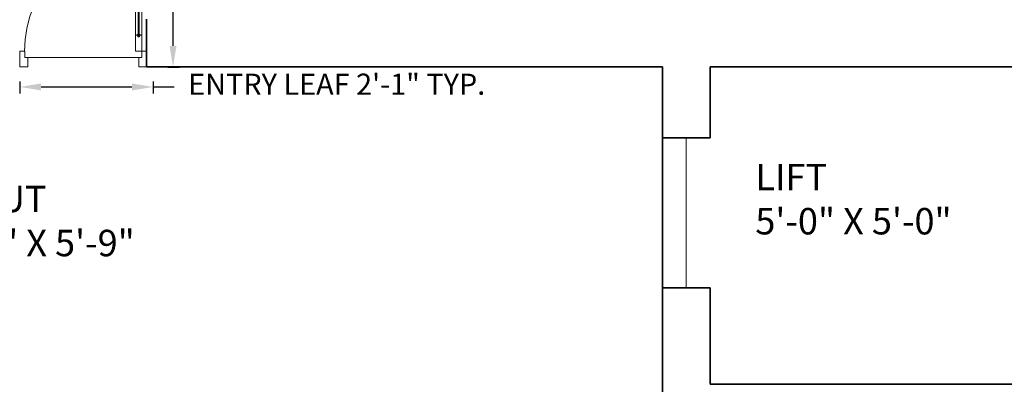
# Model space of a CAD drawing. Units: inches. Extents: x -638 to 186, y -762 to 59.
# Tile 3 of 31: x -287 to -100, y -608 to -539. Entities that reach past the tile are written whole.
import ezdxf

# ---------------------------------------------------------------- set-up
doc = ezdxf.new("R2010")
doc.units = ezdxf.units.IN
for name, color, linetype, lineweight in [('A-ANNO-DIMS', 2, 'Continuous', 18), ('A-AREA-IDEN', 1, 'Continuous', 18), ('A-DOOR', 3, 'Continuous', 18), ('wall', 7, 'Continuous', 35)]:
    doc.layers.add(name, color=color, linetype=linetype, lineweight=lineweight)
doc.styles.get("Standard").update_dxf_attribs({"font": 'arial.ttf'})
doc.dimstyles.new('ISO-25', dxfattribs={"dimtxt": 4, "dimasz": 4, "dimexe": 1.25, "dimexo": 0.625, "dimtad": 0, "dimlunit": 4, "dimtxsty": 'Standard', "dimcen": 2.5, "dimclrt": 256, "dimadec": 0, "dimazin": 0, "dimtfac": 1, "dimtmove": 0, "dimatfit": 3, "dimfxl": 1, "dimfxlon": 1, "dimarcsym": 0})

# ---------------------------------------------------------------- blocks, each defined once
blk = doc.blocks.new('DOOR-ENTRY-24IN-LEAF')
for p, q in [((22.38, 22.44), (22.37, 5.69)), ((22.45, 22.44), (22.45, 5.69)), ((22.53, 22.44), (22.52, 5.69)), ((21.85, 22.14), (21.85, 5.99)), ((23.05, 22.14), (23.04, 5.99)), ((1.5, 1.8), (22.44, 1.8))]:
    blk.add_line(p, q)
for points in [[(21.11, 23.03), (19.91, 22.91, -0.443716), (19.75, 23.06), (19.75, 24.22, -0.443716), (19.91, 24.37), (21.11, 24.25, -0.385314), (21.24, 24.1), (21.24, 23.18, -0.385314)], [(23.79, 23.03), (24.99, 22.91, 0.443716), (25.15, 23.06), (25.16, 24.22, 0.443716), (24.99, 24.37), (23.79, 24.25, 0.385314), (23.66, 24.1), (23.66, 23.18, 0.385314)]]:
    blk.add_lwpolyline(points, format="xyb", close=True)
for points in [[(22.3, 22.14), (21.85, 22.14), (21.85, 25.14), (23.05, 25.14), (23.05, 22.14), (22.6, 22.14), (22.6, 22.44), (22.3, 22.44), (22.3, 22.14)], [(22.3, 5.99), (21.85, 5.99), (21.85, 2.99), (23.04, 2.99), (23.04, 5.99), (22.59, 5.99), (22.59, 5.69), (22.3, 5.69), (22.3, 5.99)], [(0.9, 3), (0.9, 1.8), (1.5, 1.8), (1.5, 0.01), (0, 0.01), (0, 3), (0.9, 3)], [(23.04, 2.99), (23.04, 1.8), (22.44, 1.8), (22.44, 0), (23.94, 0), (23.94, 2.99), (23.04, 2.99)]]:
    blk.add_lwpolyline(points)
for points in [[(21.85, 23.49), (21.24, 23.49), (21.24, 23.79), (21.85, 23.79)], [(23.05, 23.49), (23.66, 23.49), (23.66, 23.79), (23.05, 23.79)]]:
    blk.add_lwpolyline(points, close=True)
for centre, radius, start, end in [((23.1, 2.97), 22.21, 93.2293, 179.917), ((22.36, 22.17), 0.247, 186.4162, 273.2718), ((22.54, 22.17), 0.247, 266.6922, 353.5478), ((22.36, 5.96), 0.247, 86.6922, 173.5478), ((22.53, 5.96), 0.247, 6.4162, 93.2718)]:
    blk.add_arc(centre, radius, start, end)
blk = doc.blocks.new('*D29')
at = {"layer": 'A-ANNO-DIMS', "color": 0, "lineweight": -2, "transparency": 16777216}
for p, q in [((-286.47, -550.82), (-286.47, -553.07)), ((-261.32, -550.82), (-261.32, -553.07)), ((-282.47, -551.82), (-265.32, -551.82)), ((-261.32, -551.82), (-257.32, -551.82))]:
    blk.add_line(p, q, dxfattribs=at)
at = {"layer": 'A-ANNO-DIMS', "color": 0, "lineweight": 30, "transparency": 16777216}
for points in [[(-282.47, -551.15), (-282.47, -552.49), (-286.47, -551.82)], [(-265.32, -551.15), (-265.32, -552.49), (-261.32, -551.82)]]:
    blk.add_solid(points, dxfattribs=at)
at = {"layer": 'Defpoints', "color": 0, "lineweight": 30, "transparency": 16777216}
for p in [(-286.47, -548.05), (-261.32, -548.05), (-261.32, -551.82)]:
    blk.add_point(p, dxfattribs=at)
at = {"layer": 'A-ANNO-DIMS', "transparency": 16777216, "insert": (-226.6, -551.82), "char_height": 4, "attachment_point": 5}
blk.add_mtext('ENTRY LEAF 2\'-1" TYP.', dxfattribs=at)
blk = doc.blocks.new('*D30')
at = {"layer": 'A-ANNO-DIMS', "color": 0, "lineweight": -2, "transparency": 16777216}
for p, q in [((-257.54, -522.91), (-257.54, -518.91)), ((-258.54, -522.91), (-256.29, -522.91)), ((-257.54, -544.05), (-257.54, -526.91)), ((-258.54, -548.05), (-256.29, -548.05))]:
    blk.add_line(p, q, dxfattribs=at)
at = {"layer": 'A-ANNO-DIMS', "color": 0, "lineweight": 30, "transparency": 16777216}
for points in [[(-258.21, -526.91), (-256.88, -526.91), (-257.54, -522.91)], [(-258.21, -544.05), (-256.88, -544.05), (-257.54, -548.05)]]:
    blk.add_solid(points, dxfattribs=at)
at = {"layer": 'Defpoints', "color": 0, "lineweight": 30, "transparency": 16777216}
for p in [(-261.32, -522.91), (-257.54, -522.91), (-261.32, -548.05)]:
    blk.add_point(p, dxfattribs=at)
at = {"layer": 'A-ANNO-DIMS', "transparency": 16777216, "insert": (-257.54, -506.06), "char_height": 4, "attachment_point": 5, "rotation": 90}
blk.add_mtext('2\'-1" TYP.', dxfattribs=at)
blk = doc.blocks.new('*D39')
at = {"layer": 'A-ANNO-DIMS', "color": 0, "lineweight": -2, "transparency": 16777216}
for p, q in [((-344.53, -751.58), (-344.53, -753.83)), ((-271.53, -751.58), (-271.53, -753.83)), ((-340.53, -752.58), (-313.98, -752.58)), ((-275.53, -752.58), (-302.07, -752.58))]:
    blk.add_line(p, q, dxfattribs=at)
at = {"layer": 'A-ANNO-DIMS', "color": 0, "lineweight": 30, "transparency": 16777216}
for points in [[(-340.53, -751.92), (-340.53, -753.25), (-344.53, -752.58)], [(-275.53, -751.92), (-275.53, -753.25), (-271.53, -752.58)]]:
    blk.add_solid(points, dxfattribs=at)
at = {"layer": 'Defpoints', "color": 0, "lineweight": 30, "transparency": 16777216}
for p in [(-344.53, -214.53), (-271.53, -214.53), (-271.53, -752.58)]:
    blk.add_point(p, dxfattribs=at)
at = {"layer": 'A-ANNO-DIMS', "transparency": 16777216, "insert": (-308.03, -752.58), "char_height": 4, "attachment_point": 5}
blk.add_mtext('6\'-1"', dxfattribs=at)
blk = doc.blocks.new('*D50')
at = {"layer": 'A-ANNO-DIMS', "color": 0, "lineweight": -2, "transparency": 16777216}
for p, q in [((-631.93, -557.43), (-631.93, -553.43)), ((-630.93, -561.43), (-633.18, -561.43)), ((-631.93, -561.43), (-631.93, -564.98)), ((-631.93, -589.8), (-631.93, -586.25)), ((-630.93, -589.8), (-633.18, -589.8)), ((-631.93, -593.8), (-631.93, -597.8))]:
    blk.add_line(p, q, dxfattribs=at)
at = {"layer": 'A-ANNO-DIMS', "color": 0, "lineweight": 30, "transparency": 16777216}
for points in [[(-632.59, -557.43), (-631.26, -557.43), (-631.93, -561.43)], [(-632.59, -593.8), (-631.26, -593.8), (-631.93, -589.8)]]:
    blk.add_solid(points, dxfattribs=at)
at = {"layer": 'Defpoints', "color": 0, "lineweight": 30, "transparency": 16777216}
for p in [(-156.03, -561.43), (-631.93, -589.8), (-156.03, -589.8)]:
    blk.add_point(p, dxfattribs=at)
at = {"layer": 'A-ANNO-DIMS', "transparency": 16777216, "insert": (-631.93, -575.62), "char_height": 4, "attachment_point": 5, "rotation": 90}
blk.add_mtext('2\'-4 1/2"', dxfattribs=at)
blk = doc.blocks.new('*D52')
at = {"layer": 'A-ANNO-DIMS', "color": 0, "lineweight": -2, "transparency": 16777216}
for p, q in [((-630.93, -580.03), (-633.18, -580.03)), ((-631.93, -584.03), (-631.93, -588.06)), ((-631.93, -604.03), (-631.93, -600.01)), ((-630.93, -608.03), (-633.18, -608.03))]:
    blk.add_line(p, q, dxfattribs=at)
at = {"layer": 'A-ANNO-DIMS', "color": 0, "lineweight": 30, "transparency": 16777216}
for points in [[(-632.59, -584.03), (-631.26, -584.03), (-631.93, -580.03)], [(-632.59, -604.03), (-631.26, -604.03), (-631.93, -608.03)]]:
    blk.add_solid(points, dxfattribs=at)
at = {"layer": 'Defpoints', "color": 0, "lineweight": 30, "transparency": 16777216}
for p in [(-29.91, -580.03), (-631.93, -608.03), (-40.41, -608.03)]:
    blk.add_point(p, dxfattribs=at)
at = {"layer": 'A-ANNO-DIMS', "transparency": 16777216, "insert": (-631.93, -594.03), "char_height": 4, "attachment_point": 5, "rotation": 90}
blk.add_mtext('2\'-4"', dxfattribs=at)
blk = doc.blocks.new('*D57')
at = {"layer": 'A-ANNO-DIMS', "color": 0, "lineweight": -2, "transparency": 16777216}
for p, q in [((-630.93, -548.03), (-633.18, -548.03)), ((-631.93, -552.03), (-631.93, -557.43)), ((-630.93, -561.43), (-633.18, -561.43)), ((-631.93, -561.43), (-631.93, -565.43))]:
    blk.add_line(p, q, dxfattribs=at)
at = {"layer": 'A-ANNO-DIMS', "color": 0, "lineweight": 30, "transparency": 16777216}
for points in [[(-632.59, -552.03), (-631.26, -552.03), (-631.93, -548.03)], [(-632.59, -557.43), (-631.26, -557.43), (-631.93, -561.43)]]:
    blk.add_solid(points, dxfattribs=at)
at = {"layer": 'Defpoints', "color": 0, "lineweight": 30, "transparency": 16777216}
for p in [(-156.03, -548.03), (-631.93, -561.43), (-156.03, -561.43)]:
    blk.add_point(p, dxfattribs=at)
at = {"layer": 'A-ANNO-DIMS', "transparency": 16777216, "insert": (-631.93, -575.84), "char_height": 4, "attachment_point": 5, "rotation": 90}
blk.add_mtext('1\'-1 1/2"', dxfattribs=at)

msp = doc.modelspace()

# ---------------------------------------------------------------- linework, layer by layer
at = {"layer": 'A-DOOR'}
msp.add_line((-160.526, -561.427), (-160.526, -589.804), dxfattribs=at)
at = {"layer": 'wall'}
for p, q in [((-262.526, -539.033), (-262.526, -548.033)), ((-165.026, -548.033), (-262.526, -548.033)), ((-165.026, -548.033), (-165.026, -608.033)), ((-156.026, -548.033), (-96.026, -548.033)), ((-156.026, -548.033), (-156.026, -557.033)), ((-156.026, -557.033), (-156.026, -561.427)), ((-156.026, -561.427), (-165.026, -561.427)), ((-156.026, -589.804), (-165.026, -589.804)), ((-156.026, -608.033), (-156.026, -589.804)), ((-165.026, -608.033), (-165.026, -617.033)), ((-96.026, -608.033), (-156.026, -608.033))]:
    msp.add_line(p, q, dxfattribs=at)

# ---------------------------------------------------------------- block references
at = {"layer": 'A-DOOR'}
msp.add_blockref('DOOR-ENTRY-24IN-LEAF', (-286.471, -548.048), dxfattribs=at)

# ---------------------------------------------------------------- texts
at = {"layer": 'A-AREA-IDEN', "char_height": 5, "attachment_point": 1}
for s, width, insert in [('\\A1;{LIFT\\P5\'-0" X 5\'-0\\H1x;"}', 99.04816, (-147.474, -566.364)), ('SITOUT\\P20\'-8" X 5\'-9"', 91.13387, (-305.654, -570.49))]:
    msp.add_mtext_dynamic_manual_height_columns(s, width=width, gutter_width=12.5, heights=[0], dxfattribs=dict(at, insert=insert))

# ---------------------------------------------------------------- dimensions: what is measured, and where the dimension line sits
at = {"layer": 'A-ANNO-DIMS'}
dim = msp.add_linear_dim(base=(-271.526, -752.583), p1=(-344.526, -214.533), p2=(-271.526, -214.533), dimstyle='ISO-25', override={"dimdec": 1, "dimlfac": 1, "dimrnd": 0, "dimzin": 1, "dimdsep": 46, "dimlunit": 4, "dimfrac": 2}, dxfattribs=at)
dim.commit()
dim.dimension.update_dxf_attribs({"geometry": '*D39', "text_midpoint": (-308.026, -752.583)})
dim = msp.add_linear_dim(base=(-257.543, -522.911), p1=(-261.316, -548.048), p2=(-261.316, -522.911), angle=90, text='<> TYP.', dimstyle='ISO-25', override={"dimdec": 1, "dimlfac": 1, "dimrnd": 0, "dimzin": 1, "dimdsep": 46, "dimlunit": 4, "dimfrac": 2}, dxfattribs=at)
dim.commit()
dim.dimension.update_dxf_attribs({"geometry": '*D30', "text_midpoint": (-257.543, -506.061)})
dim = msp.add_linear_dim(base=(-261.316, -551.822), p1=(-286.471, -548.048), p2=(-261.316, -548.048), text='ENTRY LEAF <> TYP.', dimstyle='ISO-25', override={"dimdec": 1, "dimlfac": 1, "dimrnd": 0, "dimzin": 1, "dimdsep": 46, "dimlunit": 4, "dimfrac": 2}, dxfattribs=at)
dim.commit()
dim.dimension.update_dxf_attribs({"geometry": '*D29', "text_midpoint": (-226.596, -551.822)})
for base, p1, p2, picture, middle in [((-631.926, -561.427), (-156.026, -548.033), (-156.026, -561.427), '*D57', (-631.926, -575.84)), ((-631.926, -589.804), (-156.026, -561.427), (-156.026, -589.804), '*D50', (-631.926, -575.615)), ((-631.926, -608.033), (-29.908, -580.033), (-40.408, -608.033), '*D52', (-631.926, -594.033))]:
    dim = msp.add_linear_dim(base=base, p1=p1, p2=p2, angle=90, dimstyle='ISO-25', override={"dimdec": 1, "dimlfac": 1, "dimrnd": 0, "dimzin": 1, "dimdsep": 46, "dimlunit": 4, "dimfrac": 2}, dxfattribs=at)
    dim.commit()
    dim.dimension.update_dxf_attribs({"geometry": picture, "text_midpoint": middle})

doc.saveas('drawing.dxf')
